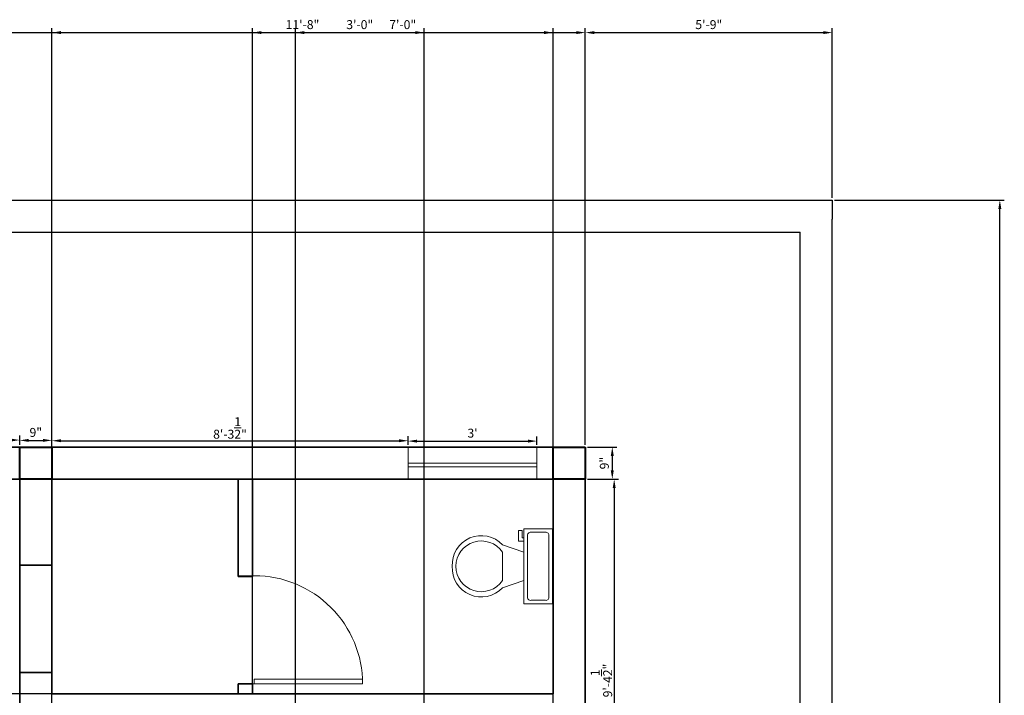
# Model space of a CAD drawing. Units: inches. Extents: x 1624 to 3956, y 1589 to 5028.
# Tile 16 of 16: x 1943 to 2218, y 2426 to 2615. Entities that reach past the tile are written whole.
import ezdxf

# ---------------------------------------------------------------- set-up
doc = ezdxf.new("R2010")
doc.units = ezdxf.units.IN
for name, color, linetype, lineweight in [('A-ANNO-DIMS', 2, 'Continuous', 13), ('A-COLS', 1, 'Continuous', 40), ('A-DOOR', 3, 'Continuous', 18), ('A-FLOR-FIXT', 9, 'Continuous', 18), ('A-GLAZ', 4, 'Continuous', 18), ('A-WALL', 7, 'Continuous', 35), ('C-PROP', 7, 'Continuous', 25)]:
    doc.layers.add(name, color=color, linetype=linetype, lineweight=lineweight)
doc.styles.get("Standard").update_dxf_attribs({"font": 'arial.ttf'})
doc.dimstyles.new('Copy of ISO-25', dxfattribs={"dimtxt": 2.5, "dimasz": 2.5, "dimexe": 1.25, "dimexo": 0.625, "dimtad": 1, "dimdec": 1, "dimlunit": 4, "dimtxsty": 'Standard', "dimcen": 2.5, "dimadec": 0, "dimazin": 0, "dimtfac": 1, "dimtdec": 1, "dimtmove": 0, "dimatfit": 3, "dimfxl": 1, "dimarcsym": 0})

# ---------------------------------------------------------------- blocks, each defined once
blk = doc.blocks.new('*U5')
for p, q in [((0, 0), (0, 6)), ((40, 0), (40, 6))]:
    blk.add_line(p, q)
blk.add_lwpolyline([(0, 0), (0, -40), (1.75, -40), (1.75, 0)], close=True)
blk.add_arc((0, 0), 40, 270, 0)
blk = doc.blocks.new('*U14')
for p, q in [((241.3, -152.4), (241.3, -50.8)), ((-203.2, -215.9), (-203.2, -203.2)), ((-177.8, -203.2), (-177.8, -241.3)), ((-101.6, -203.2), (-152.4, -355.6)), ((101.6, -203.2), (152.4, -355.6)), ((-254, -215.9), (-203.2, -215.9)), ((-254, -241.3), (-254, -215.9)), ((-177.8, -241.3), (-254, -241.3)), ((101.6, -355.6), (-101.6, -355.6))]:
    blk.add_line(p, q)
blk.add_lwpolyline([(266.7, -203.2), (266.7, 0), (-266.7, 0), (-266.7, -203.2)], close=True)
for points in [[(-241.3, -50.8), (-241.3, -152.4)], [(215.9, -25.4), (-215.9, -25.4)], [(-215.9, -177.8), (215.9, -177.8)]]:
    blk.add_lwpolyline(points)
for centre, radius, start, end in [((-219.075, -47.625), 22.45064, 81.8699, 188.1301), ((219.075, -47.625), 22.45064, 351.8699, 98.1301), ((-219.075, -155.575), 22.45064, 171.869898, 278.1301), ((219.075, -155.575), 22.45064, 261.8699, 8.1301), ((-12.12088, -505.93752), 205.61935, 133.01722, 273.38), ((0.94996, -504.77674), 181.02486, 124.50543, 269.7), ((-0.94742, -504.77674), 181.02486, 270.3, 55.4946), ((12.12342, -505.93752), 205.61935, 266.62, 46.9828)]:
    blk.add_arc(centre, radius, start, end)
blk = doc.blocks.new('*D30')
at = {"layer": 'A-ANNO-DIMS', "color": 0, "lineweight": -2, "transparency": 16777216}
for p, q in [((1908.58, 2496.42), (1908.58, 2498.98)), ((1911.08, 2497.73), (1940.08, 2497.73)), ((1942.58, 2496.42), (1942.58, 2498.98))]:
    blk.add_line(p, q, dxfattribs=at)
at = {"layer": 'A-ANNO-DIMS', "color": 0, "transparency": 16777216}
for points in [[(1911.08, 2498.14), (1911.08, 2497.31), (1908.58, 2497.73)], [(1940.08, 2498.14), (1940.08, 2497.31), (1942.58, 2497.73)]]:
    blk.add_solid(points, dxfattribs=at)
at = {"layer": 'Defpoints', "color": 0, "transparency": 16777216}
for p in [(1942.58, 2497.73), (1908.58, 2495.79), (1942.58, 2495.79)]:
    blk.add_point(p, dxfattribs=at)
at = {"layer": 'A-ANNO-DIMS', "color": 0, "transparency": 16777216, "insert": (1925.58, 2499.63), "char_height": 2.5, "attachment_point": 5}
blk.add_mtext('2\'-10"', dxfattribs=at)
blk = doc.blocks.new('*D31')
at = {"layer": 'A-ANNO-DIMS', "color": 0, "lineweight": -2, "transparency": 16777216}
for p, q in [((1942.58, 2496.42), (1942.58, 2498.89)), ((1945.08, 2497.64), (1949.08, 2497.64)), ((1951.58, 2496.42), (1951.58, 2498.89))]:
    blk.add_line(p, q, dxfattribs=at)
at = {"layer": 'A-ANNO-DIMS', "color": 0, "transparency": 16777216}
for points in [[(1945.08, 2498.06), (1945.08, 2497.22), (1942.58, 2497.64)], [(1949.08, 2498.06), (1949.08, 2497.22), (1951.58, 2497.64)]]:
    blk.add_solid(points, dxfattribs=at)
at = {"layer": 'Defpoints', "color": 0, "transparency": 16777216}
for p in [(1951.58, 2497.64), (1942.58, 2495.79), (1951.58, 2495.79)]:
    blk.add_point(p, dxfattribs=at)
at = {"layer": 'A-ANNO-DIMS', "color": 0, "transparency": 16777216, "insert": (1947.08, 2499.54), "char_height": 2.5, "attachment_point": 5}
blk.add_mtext('9"', dxfattribs=at)
blk = doc.blocks.new('*D32')
at = {"layer": 'A-ANNO-DIMS', "color": 0, "lineweight": -2, "transparency": 16777216}
for p, q in [((1951.58, 2496.42), (1951.58, 2498.79)), ((1954.08, 2497.54), (2048.58, 2497.54)), ((2051.08, 2496.42), (2051.08, 2498.79))]:
    blk.add_line(p, q, dxfattribs=at)
at = {"layer": 'A-ANNO-DIMS', "color": 0, "transparency": 16777216}
for points in [[(1954.08, 2497.96), (1954.08, 2497.13), (1951.58, 2497.54)], [(2048.58, 2497.96), (2048.58, 2497.13), (2051.08, 2497.54)]]:
    blk.add_solid(points, dxfattribs=at)
at = {"layer": 'Defpoints', "color": 0, "transparency": 16777216}
for p in [(2051.08, 2497.54), (1951.58, 2495.79), (2051.08, 2495.79)]:
    blk.add_point(p, dxfattribs=at)
at = {"layer": 'A-ANNO-DIMS', "color": 0, "transparency": 16777216, "insert": (2001.33, 2501.12), "char_height": 2.5, "attachment_point": 5}
blk.add_mtext('8\'-3{\\H1x;\\S1/2;}"', dxfattribs=at)
blk = doc.blocks.new('*D33')
at = {"layer": 'A-ANNO-DIMS', "color": 0, "lineweight": -2, "transparency": 16777216}
for p, q in [((2051.08, 2496.42), (2051.08, 2498.69)), ((2087.08, 2496.42), (2087.08, 2498.69)), ((2053.58, 2497.44), (2084.58, 2497.44))]:
    blk.add_line(p, q, dxfattribs=at)
at = {"layer": 'A-ANNO-DIMS', "color": 0, "transparency": 16777216}
for points in [[(2053.58, 2497.85), (2053.58, 2497.02), (2051.08, 2497.44)], [(2084.58, 2497.85), (2084.58, 2497.02), (2087.08, 2497.44)]]:
    blk.add_solid(points, dxfattribs=at)
at = {"layer": 'Defpoints', "color": 0, "transparency": 16777216}
for p in [(2051.08, 2495.79), (2087.08, 2497.44), (2087.08, 2495.79)]:
    blk.add_point(p, dxfattribs=at)
at = {"layer": 'A-ANNO-DIMS', "color": 0, "transparency": 16777216, "insert": (2069.08, 2499.34), "char_height": 2.5, "attachment_point": 5}
blk.add_mtext("3'", dxfattribs=at)
blk = doc.blocks.new('*D34')
at = {"layer": 'A-ANNO-DIMS', "color": 0, "lineweight": -2, "transparency": 16777216}
for p, q in [((2101.2, 2495.79), (2109.37, 2495.79)), ((2108.12, 2493.29), (2108.12, 2489.29)), ((2101.2, 2486.79), (2109.37, 2486.79))]:
    blk.add_line(p, q, dxfattribs=at)
at = {"layer": 'A-ANNO-DIMS', "color": 0, "transparency": 16777216}
for points in [[(2107.7, 2493.29), (2108.53, 2493.29), (2108.12, 2495.79)], [(2107.7, 2489.29), (2108.53, 2489.29), (2108.12, 2486.79)]]:
    blk.add_solid(points, dxfattribs=at)
at = {"layer": 'Defpoints', "color": 0, "transparency": 16777216}
for p in [(2100.58, 2495.79), (2100.58, 2486.79), (2108.12, 2486.79)]:
    blk.add_point(p, dxfattribs=at)
at = {"layer": 'A-ANNO-DIMS', "color": 0, "transparency": 16777216, "insert": (2106.22, 2491.29), "char_height": 2.5, "attachment_point": 5, "rotation": 90}
blk.add_mtext('9"', dxfattribs=at)
blk = doc.blocks.new('*D35')
at = {"layer": 'A-ANNO-DIMS', "color": 0, "lineweight": -2, "transparency": 16777216}
for p, q in [((2101.2, 2486.79), (2109.9, 2486.79)), ((2108.65, 2484.29), (2108.65, 2376.79)), ((2101.2, 2374.29), (2109.9, 2374.29))]:
    blk.add_line(p, q, dxfattribs=at)
at = {"layer": 'A-ANNO-DIMS', "color": 0, "transparency": 16777216}
for points in [[(2108.23, 2484.29), (2109.07, 2484.29), (2108.65, 2486.79)], [(2108.23, 2376.79), (2109.07, 2376.79), (2108.65, 2374.29)]]:
    blk.add_solid(points, dxfattribs=at)
at = {"layer": 'Defpoints', "color": 0, "transparency": 16777216}
for p in [(2100.58, 2486.79), (2100.58, 2374.29), (2108.65, 2374.29)]:
    blk.add_point(p, dxfattribs=at)
at = {"layer": 'A-ANNO-DIMS', "color": 0, "transparency": 16777216, "insert": (2105.08, 2430.54), "char_height": 2.5, "attachment_point": 5, "rotation": 90}
blk.add_mtext('9\'-4{\\H1x;\\S1/2;}"', dxfattribs=at)
blk = doc.blocks.new('COLUMN-9x9')
for p, q in [((0, 0), (0, 9)), ((0, 9), (9, 9)), ((9, 9), (9, 0)), ((9, 0), (0, 0))]:
    blk.add_line(p, q)
blk = doc.blocks.new('WINDOW-36IN')
for p, q in [((0, 0), (0, 9)), ((36, 9), (36, 0)), ((0, 4.5), (36, 4.5)), ((0, 3.5), (36, 3.5))]:
    blk.add_line(p, q)
blk = doc.blocks.new('*D67')
at = {"layer": 'A-ANNO-DIMS', "color": 0, "lineweight": -2, "transparency": 16777216}
for p, q in [((2170.2, 2564.79), (2217.63, 2564.79)), ((2216.38, 1649.29), (2216.38, 2562.29)), ((2170.2, 1646.79), (2217.63, 1646.79))]:
    blk.add_line(p, q, dxfattribs=at)
at = {"layer": 'A-ANNO-DIMS', "color": 0, "transparency": 16777216}
for points in [[(2215.96, 2562.29), (2216.8, 2562.29), (2216.38, 2564.79)], [(2215.96, 1649.29), (2216.8, 1649.29), (2216.38, 1646.79)]]:
    blk.add_solid(points, dxfattribs=at)
at = {"layer": 'Defpoints', "color": 0, "transparency": 16777216}
for p in [(2169.58, 2564.79), (2216.38, 2564.79), (2169.58, 1646.79)]:
    blk.add_point(p, dxfattribs=at)
at = {"layer": 'A-ANNO-DIMS', "color": 0, "transparency": 16777216, "insert": (2214.48, 2105.79), "char_height": 2.5, "attachment_point": 5, "rotation": 90}
blk.add_mtext('76\'-6"', dxfattribs=at)
blk = doc.blocks.new('*D68')
at = {"layer": 'A-ANNO-DIMS', "color": 0, "lineweight": -2, "transparency": 16777216}
for p, q in [((1728.58, 2496.42), (1728.58, 2612.84)), ((1731.08, 2611.59), (2098.08, 2611.59)), ((2100.58, 2496.42), (2100.58, 2612.84))]:
    blk.add_line(p, q, dxfattribs=at)
at = {"layer": 'A-ANNO-DIMS', "color": 0, "transparency": 16777216}
for points in [[(1731.08, 2612.01), (1731.08, 2611.18), (1728.58, 2611.59)], [(2098.08, 2612.01), (2098.08, 2611.18), (2100.58, 2611.59)]]:
    blk.add_solid(points, dxfattribs=at)
at = {"layer": 'Defpoints', "color": 0, "transparency": 16777216}
for p in [(2100.58, 2611.59), (1728.58, 2495.79), (2100.58, 2495.79)]:
    blk.add_point(p, dxfattribs=at)
at = {"layer": 'A-ANNO-DIMS', "color": 0, "transparency": 16777216, "insert": (1914.58, 2613.5), "char_height": 2.5, "attachment_point": 5}
blk.add_mtext('31\'-0"', dxfattribs=at)
blk = doc.blocks.new('*D72')
at = {"layer": 'A-ANNO-DIMS', "color": 0, "lineweight": -2, "transparency": 16777216}
for p, q in [((2100.58, 2496.42), (2100.58, 2612.84)), ((2103.08, 2611.59), (2167.08, 2611.59)), ((2169.58, 2565.42), (2169.58, 2612.84))]:
    blk.add_line(p, q, dxfattribs=at)
at = {"layer": 'A-ANNO-DIMS', "color": 0, "transparency": 16777216}
for points in [[(2103.08, 2612.01), (2103.08, 2611.18), (2100.58, 2611.59)], [(2167.08, 2612.01), (2167.08, 2611.18), (2169.58, 2611.59)]]:
    blk.add_solid(points, dxfattribs=at)
at = {"layer": 'Defpoints', "color": 0, "transparency": 16777216}
for p in [(2169.58, 2611.59), (2169.58, 2564.79), (2100.58, 2495.79)]:
    blk.add_point(p, dxfattribs=at)
at = {"layer": 'A-ANNO-DIMS', "color": 0, "transparency": 16777216, "insert": (2135.08, 2613.5), "char_height": 2.5, "attachment_point": 5}
blk.add_mtext('5\'-9"', dxfattribs=at)
blk = doc.blocks.new('*D81')
at = {"layer": 'A-ANNO-DIMS', "color": 0, "lineweight": -2, "transparency": 16777216}
for p, q in [((1951.58, 2254.92), (1951.58, 2612.84)), ((1954.08, 2611.59), (2089.08, 2611.59)), ((2091.58, 2254.92), (2091.58, 2612.84))]:
    blk.add_line(p, q, dxfattribs=at)
at = {"layer": 'A-ANNO-DIMS', "color": 0, "transparency": 16777216}
for points in [[(1954.08, 2612.01), (1954.08, 2611.18), (1951.58, 2611.59)], [(2089.08, 2612.01), (2089.08, 2611.18), (2091.58, 2611.59)]]:
    blk.add_solid(points, dxfattribs=at)
at = {"layer": 'Defpoints', "color": 0, "transparency": 16777216}
for p in [(2091.58, 2611.59), (1951.58, 2254.29), (2091.58, 2254.29)]:
    blk.add_point(p, dxfattribs=at)
at = {"layer": 'A-ANNO-DIMS', "color": 0, "transparency": 16777216, "insert": (2021.58, 2613.5), "char_height": 2.5, "attachment_point": 5}
blk.add_mtext('11\'-8"', dxfattribs=at)
blk = doc.blocks.new('*D88')
at = {"layer": 'A-ANNO-DIMS', "color": 0, "lineweight": -2, "transparency": 16777216}
for p, q in [((2007.58, 2427.42), (2007.58, 2612.84)), ((2010.08, 2611.59), (2089.08, 2611.59)), ((2091.58, 2427.42), (2091.58, 2612.84))]:
    blk.add_line(p, q, dxfattribs=at)
at = {"layer": 'A-ANNO-DIMS', "color": 0, "transparency": 16777216}
for points in [[(2010.08, 2612.01), (2010.08, 2611.18), (2007.58, 2611.59)], [(2089.08, 2612.01), (2089.08, 2611.18), (2091.58, 2611.59)]]:
    blk.add_solid(points, dxfattribs=at)
at = {"layer": 'Defpoints', "color": 0, "transparency": 16777216}
for p in [(2091.58, 2611.59), (2007.58, 2426.79), (2091.58, 2426.79)]:
    blk.add_point(p, dxfattribs=at)
at = {"layer": 'A-ANNO-DIMS', "color": 0, "transparency": 16777216, "insert": (2049.58, 2613.5), "char_height": 2.5, "attachment_point": 5}
blk.add_mtext('7\'-0"', dxfattribs=at)
blk = doc.blocks.new('*D89')
at = {"layer": 'A-ANNO-DIMS', "color": 0, "lineweight": -2, "transparency": 16777216}
for p, q in [((2090.95, 2486.79), (1628.86, 2486.79)), ((1630.11, 2484.29), (1630.11, 2429.29)), ((2090.95, 2426.79), (1628.86, 2426.79))]:
    blk.add_line(p, q, dxfattribs=at)
at = {"layer": 'A-ANNO-DIMS', "color": 0, "transparency": 16777216}
for points in [[(1629.69, 2484.29), (1630.53, 2484.29), (1630.11, 2486.79)], [(1629.69, 2429.29), (1630.53, 2429.29), (1630.11, 2426.79)]]:
    blk.add_solid(points, dxfattribs=at)
at = {"layer": 'Defpoints', "color": 0, "transparency": 16777216}
for p in [(2091.58, 2486.79), (1630.11, 2426.79), (2091.58, 2426.79)]:
    blk.add_point(p, dxfattribs=at)
at = {"layer": 'A-ANNO-DIMS', "color": 0, "transparency": 16777216, "insert": (1628.21, 2456.79), "char_height": 2.5, "attachment_point": 5, "rotation": 90}
blk.add_mtext('5\'-0"', dxfattribs=at)
blk = doc.blocks.new('*D90')
at = {"layer": 'A-ANNO-DIMS', "color": 0, "lineweight": -2, "transparency": 16777216}
for p, q in [((2019.58, 1941.92), (2019.58, 2612.84)), ((2022.08, 2611.59), (2053.08, 2611.59)), ((2055.58, 1941.92), (2055.58, 2612.84))]:
    blk.add_line(p, q, dxfattribs=at)
at = {"layer": 'A-ANNO-DIMS', "color": 0, "transparency": 16777216}
for points in [[(2022.08, 2612.01), (2022.08, 2611.18), (2019.58, 2611.59)], [(2053.08, 2612.01), (2053.08, 2611.18), (2055.58, 2611.59)]]:
    blk.add_solid(points, dxfattribs=at)
at = {"layer": 'Defpoints', "color": 0, "transparency": 16777216}
for p in [(2055.58, 2611.59), (2019.58, 1941.29), (2055.58, 1941.29)]:
    blk.add_point(p, dxfattribs=at)
at = {"layer": 'A-ANNO-DIMS', "color": 0, "transparency": 16777216, "insert": (2037.58, 2613.5), "char_height": 2.5, "attachment_point": 5}
blk.add_mtext('3\'-0"', dxfattribs=at)

msp = doc.modelspace()

# ---------------------------------------------------------------- linework, layer by layer
at = {"layer": 'A-GLAZ'}
msp.add_line((2087.08, 2495.79), (2051.08, 2495.79), dxfattribs=at)
at = {"layer": 'A-WALL'}
for p, q in [((1913.08, 2495.79), (1947.08, 2495.79)), ((1947.08, 2495.79), (1956.08, 2495.79)), ((1956.08, 2495.79), (2055.58, 2495.79)), ((2055.58, 2495.79), (2100.58, 2495.79)), ((2100.58, 2495.79), (2091.58, 2495.79)), ((2100.58, 2495.79), (2100.58, 2486.79)), ((1942.58, 2486.79), (1798.58, 2486.79)), ((1913.08, 2486.79), (1942.58, 2486.79)), ((1942.58, 2462.79), (1942.58, 2486.79)), ((1951.58, 2486.79), (1956.08, 2486.79)), ((1951.58, 2462.79), (1951.58, 2486.79)), ((1951.58, 2486.79), (2003.58, 2486.79)), ((1956.08, 2486.79), (2055.58, 2486.79)), ((2003.58, 2486.79), (2003.58, 2459.58)), ((2007.58, 2486.79), (2007.58, 2459.58)), ((2055.58, 2486.79), (2091.58, 2486.79)), ((2091.58, 2486.79), (2087.08, 2486.79)), ((2091.58, 2486.79), (2091.58, 2426.79)), ((2091.58, 2486.79), (2091.58, 2426.79)), ((2100.58, 2486.79), (2100.58, 2374.29)), ((1951.58, 2462.79), (1942.58, 2462.79)), ((1942.58, 2462.79), (1942.58, 2432.79)), ((1951.58, 2462.79), (1951.58, 2432.79)), ((2003.58, 2459.58), (2007.58, 2459.58)), ((1942.58, 2315.79), (1942.58, 2432.79)), ((1951.58, 2432.79), (1942.58, 2432.79)), ((1951.58, 2426.79), (1951.58, 2432.79)), ((1951.58, 2428.79), (1951.58, 2432.79)), ((1951.58, 2426.79), (1951.58, 2428.79)), ((2003.58, 2426.79), (2003.58, 2429.58)), ((2003.58, 2429.58), (2007.58, 2429.58)), ((2003.58, 2429.58), (2003.58, 2426.79)), ((2007.58, 2429.58), (2007.58, 2426.79)), ((2091.58, 2426.79), (1951.58, 2426.79))]:
    msp.add_line(p, q, dxfattribs=at)
at = {"layer": 'C-PROP'}
for p, q in [((1728.58, 2564.79), (2160.58, 2564.79)), ((2160.58, 2564.79), (2169.58, 2564.79)), ((2169.58, 2564.79), (2169.58, 2559.46)), ((2169.58, 1652.79), (2169.58, 2559.46)), ((1732.58, 2555.79), (2160.58, 2555.79)), ((2160.58, 1652.79), (2160.58, 2555.79))]:
    msp.add_line(p, q, dxfattribs=at)

# ---------------------------------------------------------------- block references
at = {"layer": 'A-COLS'}
for p in [(1942.58, 2486.79), (2091.58, 2486.79)]:
    msp.add_blockref('COLUMN-9x9', p, dxfattribs=at)
at = {"layer": 'A-DOOR', "xscale": 0.7562869948231716, "yscale": 0.7562869948231716, "zscale": 0.7562869948231716, "rotation": 89.99999999999999}
msp.add_blockref('*U5', (2008.12, 2429.58), dxfattribs=at)
at = {"layer": 'A-FLOR-FIXT', "xscale": 0.0393700787401575, "yscale": 0.0393700787401575, "zscale": 0.0393700787401575, "rotation": 270}
msp.add_blockref('*U14', (2091.42, 2462.45), dxfattribs=at)
at = {"layer": 'A-GLAZ'}
msp.add_blockref('WINDOW-36IN', (2051.08, 2486.79), dxfattribs=at)

# ---------------------------------------------------------------- dimensions: what is measured, and where the dimension line sits
at = {"layer": 'A-ANNO-DIMS'}
for base, p1, p2, override, picture, middle in [((2100.58, 2611.59), (1728.58, 2495.79), (2100.58, 2495.79), {"dimdec": 1, "dimlfac": 1, "dimrnd": 0, "dimzin": 1, "dimdsep": 46, "dimlunit": 4, "dimfrac": 2}, '*D68', (1914.58, 2613.5)), ((2091.58, 2611.59), (1951.58, 2254.29), (2091.58, 2254.29), {"dimdec": 1, "dimlfac": 1, "dimrnd": 0, "dimzin": 1, "dimdsep": 46, "dimlunit": 4, "dimfrac": 2}, '*D81', (2021.58, 2613.5)), ((2091.58, 2611.59), (2007.58, 2426.79), (2091.58, 2426.79), {"dimdec": 1, "dimlfac": 1, "dimrnd": 0, "dimzin": 1, "dimdsep": 46, "dimlunit": 4, "dimfrac": 2}, '*D88', (2049.58, 2613.5)), ((2055.58, 2611.59), (2019.58, 1941.29), (2055.58, 1941.29), {"dimdec": 1, "dimlfac": 1, "dimrnd": 0, "dimzin": 1, "dimdsep": 46, "dimlunit": 4, "dimfrac": 2}, '*D90', (2037.58, 2613.5)), ((2169.58, 2611.59), (2100.58, 2495.79), (2169.58, 2564.79), {"dimdec": 1, "dimlfac": 1, "dimrnd": 0, "dimzin": 1, "dimdsep": 46, "dimlunit": 4, "dimfrac": 2}, '*D72', (2135.08, 2613.5)), ((2051.08, 2497.54), (1951.58, 2495.79), (2051.08, 2495.79), {"dimclrd": 0, "dimclre": 0, "dimclrt": 0}, '*D32', (2001.33, 2501.12)), ((1942.58, 2497.73), (1908.58, 2495.79), (1942.58, 2495.79), {"dimclrd": 0, "dimclre": 0, "dimclrt": 0}, '*D30', (1925.58, 2499.63)), ((1951.58, 2497.64), (1942.58, 2495.79), (1951.58, 2495.79), {"dimclrd": 0, "dimclre": 0, "dimclrt": 0}, '*D31', (1947.08, 2499.54)), ((2087.08, 2497.44), (2051.08, 2495.79), (2087.08, 2495.79), {"dimclrd": 0, "dimclre": 0, "dimclrt": 0}, '*D33', (2069.08, 2499.34))]:
    dim = msp.add_linear_dim(base=base, p1=p1, p2=p2, dimstyle='Copy of ISO-25', override=override, dxfattribs=at)
    dim.commit()
    dim.dimension.update_dxf_attribs({"geometry": picture, "text_midpoint": middle})
for base, p1, p2, override, picture, middle in [((2216.38, 2564.79), (2169.58, 1646.79), (2169.58, 2564.79), {"dimdec": 1, "dimlfac": 1, "dimrnd": 0, "dimzin": 1, "dimdsep": 46, "dimlunit": 4, "dimfrac": 2}, '*D67', (2214.48, 2105.79)), ((2108.12, 2486.79), (2100.58, 2495.79), (2100.58, 2486.79), {"dimclrd": 0, "dimclre": 0, "dimclrt": 0}, '*D34', (2106.22, 2491.29)), ((1630.11, 2426.79), (2091.58, 2486.79), (2091.58, 2426.79), {"dimdec": 1, "dimlfac": 1, "dimrnd": 0, "dimzin": 1, "dimdsep": 46, "dimlunit": 4, "dimfrac": 2}, '*D89', (1628.21, 2456.79)), ((2108.65, 2374.29), (2100.58, 2486.79), (2100.58, 2374.29), {"dimclrd": 0, "dimclre": 0, "dimclrt": 0}, '*D35', (2105.08, 2430.54))]:
    dim = msp.add_linear_dim(base=base, p1=p1, p2=p2, angle=90, dimstyle='Copy of ISO-25', override=override, dxfattribs=at)
    dim.commit()
    dim.dimension.update_dxf_attribs({"geometry": picture, "text_midpoint": middle})

doc.saveas('drawing.dxf')
